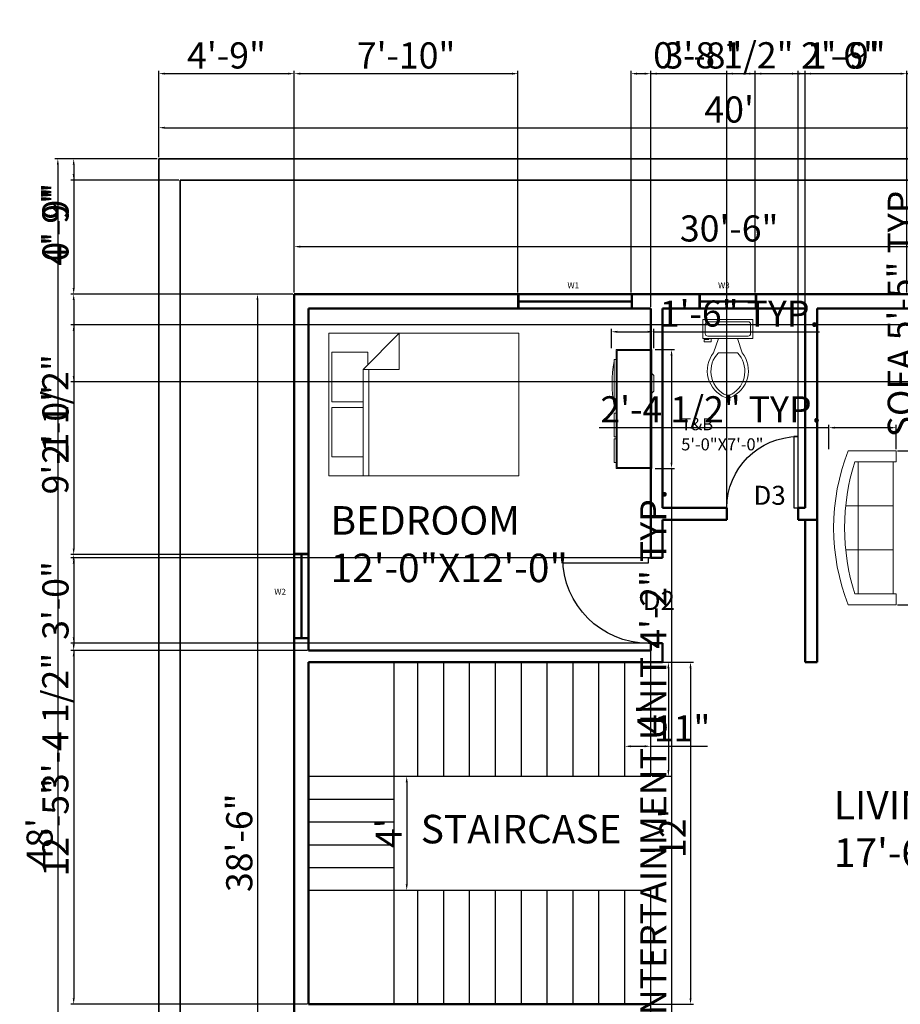
# Model space of a CAD drawing. Units: inches. Extents: x 2299 to 4423, y 1066 to 1805.
# Tile 2 of 7: x 2299 to 2670, y 1391 to 1805. Entities that reach past the tile are written whole.
import ezdxf

# ---------------------------------------------------------------- set-up
doc = ezdxf.new("R2010")
doc.units = ezdxf.units.IN
for name, color, linetype, lineweight in [('A-ANNO-DIMS', 2, 'Continuous', 18), ('A-ANNO-TEXT', 1, 'Continuous', 25), ('A-AREA-IDEN', 1, 'Continuous', 25), ('A-DOOR', 5, 'Continuous', 25), ('A-FLOR-STRS', 6, 'Continuous', 25), ('A-FURN', 8, 'Continuous', 18), ('A-GLAZ', 3, 'Continuous', 25), ('A-WALL', 7, 'Continuous', 50), ('C-PROP', 7, 'Continuous', 35)]:
    doc.layers.add(name, color=color, linetype=linetype, lineweight=lineweight)
doc.styles.get("Standard").update_dxf_attribs({"font": 'arial.ttf'})
doc.dimstyles.new('ISO-25', dxfattribs={"dimtxt": 11, "dimasz": 2.5, "dimexe": 1.25, "dimexo": 0.625, "dimtad": 1, "dimlunit": 4, "dimtxsty": 'Standard', "dimcen": 2.5, "dimadec": 0, "dimazin": 0, "dimtfac": 1, "dimtmove": 0, "dimatfit": 3, "dimfxl": 1, "dimarcsym": 0})

# ---------------------------------------------------------------- blocks, each defined once
blk = doc.blocks.new('*U2')
for p, q in [((0, 0), (0, -5)), ((30, 0), (30, -5))]:
    blk.add_line(p, q)
blk.add_lwpolyline([(0, 0), (0, 30), (1.75, 30), (1.75, 0)], close=True)
blk.add_arc((0, 0), 30, 0, 90)
blk = doc.blocks.new('Bed - Queen')
for p, q in [((0, -80.00003), (0, 0)), ((0, 0), (59.99999, 0)), ((59.99999, 0), (59.99999, -80.00003)), ((7.99999, -1.2), (28.79998, -1.2)), ((7.99999, -14.4), (7.99999, -1.2)), ((28.79998, -1.2), (28.79998, -14.4)), ((31.19999, -1.2), (51.99999, -1.2)), ((31.19999, -14.4), (31.19999, -1.2)), ((51.99999, -1.2), (51.99999, -16.4)), ((0, -14.4), (44.8, -14.4)), ((59.99999, -29.6), (44.8, -14.4)), ((44.8, -14.4), (44.8, -29.6)), ((51.99999, -16.4), (46.79936, -16.4)), ((44.8, -16.8), (0, -16.8)), ((44.8, -29.6), (59.99999, -29.6)), ((59.99999, -80.00003), (0, -80.00003))]:
    blk.add_line(p, q)
blk = doc.blocks.new('Toilet - top')
for p, q in [((9.5, -6), (9.5, -2)), ((-8, -8.5), (-8, -8)), ((-7, -8), (-7, -9.5)), ((-4, -8), (-6, -14)), ((4, -8), (6, -14)), ((-10, -8.5), (-8, -8.5)), ((-10, -9.5), (-10, -8.5)), ((-7, -9.5), (-10, -9.5)), ((4, -14), (-4, -14))]:
    blk.add_line(p, q)
blk.add_lwpolyline([(10.5, -8), (10.5, 0), (-10.5, 0), (-10.5, -8)], close=True)
for points in [[(-9.5, -2), (-9.5, -6)], [(8.5, -1), (-8.5, -1)], [(-8.5, -7), (8.5, -7)]]:
    blk.add_lwpolyline(points)
for centre, radius, start, end in [((-8.62, -1.88), 0.884, 81.8699, 188.1301), ((8.62, -1.88), 0.884, 351.8699, 98.1301), ((-8.62, -6.12), 0.884, 171.8699, 278.1301), ((8.62, -6.12), 0.884, 261.8699, 8.1301), ((3.52, -21.58), 12.17, 141.4691, 247.9714), ((4.2, -21.82), 11.33, 136.3677, 238.9468), ((-3.52, -21.58), 12.17, 292.0284, 38.5307), ((-4.2, -21.82), 11.33, 301.053, 43.6321), ((0, -27.88), 4, 245.7318, 294.2682), ((0, -29), 4, 254.8605, 285.1395)]:
    blk.add_arc(centre, radius, start, end)
blk = doc.blocks.new('Entertainment Center')
for p, q in [((-4, 0), (-5, -1)), ((4, 0), (-4, 0)), ((5, -1), (4, 0)), ((-17, -19), (-17, -1)), ((-17, -1), (43, -1)), ((-16.5, -18.5), (-16.5, -1.5)), ((-16.5, -1.5), (42.5, -1.5)), ((42.5, -1.5), (42.5, -18.5)), ((43, -1), (43, -19)), ((43, -19), (-17, -19)), ((42.5, -18.5), (-16.5, -18.5)), ((-12, -20), (-12, -19)), ((12, -19), (12, -20)), ((15, -20), (15, -19)), ((27, -19), (27, -20)), ((28, -20), (28, -19)), ((40, -19), (40, -20)), ((12, -20), (-12, -20)), ((27, -20), (15, -20)), ((40, -20), (28, -20))]:
    blk.add_line(p, q)
blk.add_arc((0, 40), 61, 259.6111, 280.3889)
blk = doc.blocks.new('Sofa - Roundback 7 ft.')
for p, q in [((-12.00002, -32.4421), (-12.00003, -6.5971)), ((11.99997, -32.4421), (11.99998, -6.5971)), ((-36.000027, -34), (-36.000027, -11.4696)), ((-35.999844, -13.3819), (35.9998, -13.3819)), ((35.99998, -34), (35.99998, -11.4696)), ((-36.000027, -32.4421), (35.99998, -32.4421))]:
    blk.add_line(p, q)
for points in [[(-36.000027, -34), (-42.000027, -34), (-42.000027, -8)], [(41.99998, -8), (41.99998, -34), (35.99998, -34)]]:
    blk.add_lwpolyline(points)
for centre, radius, start, end in [((0, -114.25), 114.25, 68.43141, 111.5686), ((-0.00001, -127.1968), 121.1968, 72.72033, 107.2797)]:
    blk.add_arc(centre, radius, start, end)
blk = doc.blocks.new('*D16')
at = {"layer": 'A-ANNO-DIMS', "color": 0, "lineweight": -2, "transparency": 16777216}
for p, q in [((2565.46, 1534.95), (2582.83, 1534.95)), ((2581.58, 1532.45), (2581.58, 1393.45)), ((2565.46, 1390.95), (2582.83, 1390.95))]:
    blk.add_line(p, q, dxfattribs=at)
at = {"layer": 'A-ANNO-DIMS', "color": 0, "transparency": 16777216}
for points in [[(2581.17, 1532.45), (2582, 1532.45), (2581.58, 1534.95)], [(2581.17, 1393.45), (2582, 1393.45), (2581.58, 1390.95)]]:
    blk.add_solid(points, dxfattribs=at)
at = {"layer": 'Defpoints', "color": 0, "transparency": 16777216}
for p in [(2564.83, 1534.95), (2564.83, 1390.95), (2581.58, 1390.95)]:
    blk.add_point(p, dxfattribs=at)
at = {"layer": 'A-ANNO-DIMS', "color": 0, "transparency": 16777216, "insert": (2575.43, 1462.95), "char_height": 11, "attachment_point": 5, "rotation": 90}
blk.add_mtext("12'", dxfattribs=at)
blk = doc.blocks.new('*D17')
at = {"layer": 'A-ANNO-DIMS', "color": 0, "lineweight": -2, "transparency": 16777216}
for p, q in [((2565.46, 1534.95), (2573.51, 1534.95)), ((2572.26, 1532.45), (2572.26, 1489.45)), ((2565.46, 1486.95), (2573.51, 1486.95))]:
    blk.add_line(p, q, dxfattribs=at)
at = {"layer": 'A-ANNO-DIMS', "color": 0, "transparency": 16777216}
for points in [[(2571.84, 1532.45), (2572.67, 1532.45), (2572.26, 1534.95)], [(2571.84, 1489.45), (2572.67, 1489.45), (2572.26, 1486.95)]]:
    blk.add_solid(points, dxfattribs=at)
at = {"layer": 'Defpoints', "color": 0, "transparency": 16777216}
for p in [(2564.83, 1534.95), (2564.83, 1486.95), (2572.26, 1486.95)]:
    blk.add_point(p, dxfattribs=at)
at = {"layer": 'A-ANNO-DIMS', "color": 0, "transparency": 16777216, "insert": (2566.13, 1510.95), "char_height": 11, "attachment_point": 5, "rotation": 90}
blk.add_mtext("4'", dxfattribs=at)
blk = doc.blocks.new('*D18')
at = {"layer": 'A-ANNO-DIMS', "color": 0, "lineweight": -2, "transparency": 16777216}
for p, q in [((2553.94, 1487.57), (2553.94, 1500.82)), ((2564.83, 1487.57), (2564.83, 1500.82)), ((2556.44, 1499.57), (2562.33, 1499.57)), ((2564.83, 1499.57), (2588.74, 1499.57))]:
    blk.add_line(p, q, dxfattribs=at)
at = {"layer": 'A-ANNO-DIMS', "color": 0, "transparency": 16777216}
for points in [[(2556.44, 1499.98), (2556.44, 1499.15), (2553.94, 1499.57)], [(2562.33, 1499.98), (2562.33, 1499.15), (2564.83, 1499.57)]]:
    blk.add_solid(points, dxfattribs=at)
at = {"layer": 'Defpoints', "color": 0, "transparency": 16777216}
for p in [(2564.83, 1499.57), (2553.94, 1486.95), (2564.83, 1486.95)]:
    blk.add_point(p, dxfattribs=at)
at = {"layer": 'A-ANNO-DIMS', "color": 0, "transparency": 16777216, "insert": (2578.04, 1505.71), "char_height": 11, "attachment_point": 5}
blk.add_mtext('11"', dxfattribs=at)
blk = doc.blocks.new('*D19')
at = {"layer": 'A-ANNO-DIMS', "color": 0, "lineweight": -2, "transparency": 16777216}
for p, q in [((2457.46, 1486.95), (2463.41, 1486.95)), ((2462.16, 1484.45), (2462.16, 1441.45)), ((2457.46, 1438.95), (2463.41, 1438.95))]:
    blk.add_line(p, q, dxfattribs=at)
at = {"layer": 'A-ANNO-DIMS', "color": 0, "transparency": 16777216}
for points in [[(2461.74, 1484.45), (2462.57, 1484.45), (2462.16, 1486.95)], [(2461.74, 1441.45), (2462.57, 1441.45), (2462.16, 1438.95)]]:
    blk.add_solid(points, dxfattribs=at)
at = {"layer": 'Defpoints', "color": 0, "transparency": 16777216}
for p in [(2456.83, 1486.95), (2456.83, 1438.95), (2462.16, 1438.95)]:
    blk.add_point(p, dxfattribs=at)
at = {"layer": 'A-ANNO-DIMS', "color": 0, "transparency": 16777216, "insert": (2456.03, 1462.95), "char_height": 11, "attachment_point": 5, "rotation": 90}
blk.add_mtext("4'", dxfattribs=at)
blk = doc.blocks.new('*D20')
at = {"layer": 'A-ANNO-DIMS', "color": 0, "lineweight": -2, "transparency": 16777216}
for p, q in [((2357.83, 1747.57), (2357.83, 1761.24)), ((2360.33, 1759.99), (2835.33, 1759.99)), ((2837.83, 1747.57), (2837.83, 1761.24))]:
    blk.add_line(p, q, dxfattribs=at)
at = {"layer": 'A-ANNO-DIMS', "color": 0, "transparency": 16777216}
for points in [[(2360.33, 1760.41), (2360.33, 1759.58), (2357.83, 1759.99)], [(2835.33, 1760.41), (2835.33, 1759.58), (2837.83, 1759.99)]]:
    blk.add_solid(points, dxfattribs=at)
at = {"layer": 'Defpoints', "color": 0, "transparency": 16777216}
for p in [(2837.83, 1759.99), (2357.83, 1746.95), (2837.83, 1746.95)]:
    blk.add_point(p, dxfattribs=at)
at = {"layer": 'A-ANNO-DIMS', "color": 0, "transparency": 16777216, "insert": (2597.83, 1766.23), "char_height": 11, "attachment_point": 5}
blk.add_mtext("40'", dxfattribs=at)
blk = doc.blocks.new('*D21')
at = {"layer": 'A-ANNO-DIMS', "color": 0, "lineweight": -2, "transparency": 16777216}
for p, q in [((2357.21, 1746.95), (2314.11, 1746.95)), ((2315.36, 1744.45), (2315.36, 1173.45)), ((2357.21, 1170.95), (2314.11, 1170.95))]:
    blk.add_line(p, q, dxfattribs=at)
at = {"layer": 'A-ANNO-DIMS', "color": 0, "transparency": 16777216}
for points in [[(2314.94, 1744.45), (2315.77, 1744.45), (2315.36, 1746.95)], [(2314.94, 1173.45), (2315.77, 1173.45), (2315.36, 1170.95)]]:
    blk.add_solid(points, dxfattribs=at)
at = {"layer": 'Defpoints', "color": 0, "transparency": 16777216}
for p in [(2357.83, 1746.95), (2315.36, 1170.95), (2357.83, 1170.95)]:
    blk.add_point(p, dxfattribs=at)
at = {"layer": 'A-ANNO-DIMS', "color": 0, "transparency": 16777216, "insert": (2309.11, 1458.95), "char_height": 11, "attachment_point": 5, "rotation": 90}
blk.add_mtext("48'", dxfattribs=at)
blk = doc.blocks.new('*D22')
at = {"layer": 'A-ANNO-DIMS', "color": 0, "lineweight": -2, "transparency": 16777216}
for p, q in [((2414.83, 1690.57), (2414.83, 1711.17)), ((2417.33, 1709.92), (2778.33, 1709.92)), ((2780.83, 1690.57), (2780.83, 1711.17))]:
    blk.add_line(p, q, dxfattribs=at)
at = {"layer": 'A-ANNO-DIMS', "color": 0, "transparency": 16777216}
for points in [[(2417.33, 1710.33), (2417.33, 1709.5), (2414.83, 1709.92)], [(2778.33, 1710.33), (2778.33, 1709.5), (2780.83, 1709.92)]]:
    blk.add_solid(points, dxfattribs=at)
at = {"layer": 'Defpoints', "color": 0, "transparency": 16777216}
for p in [(2780.83, 1709.92), (2414.83, 1689.95), (2780.83, 1689.95)]:
    blk.add_point(p, dxfattribs=at)
at = {"layer": 'A-ANNO-DIMS', "color": 0, "transparency": 16777216, "insert": (2597.83, 1716.16), "char_height": 11, "attachment_point": 5}
blk.add_mtext('30\'-6"', dxfattribs=at)
blk = doc.blocks.new('*D23')
at = {"layer": 'A-ANNO-DIMS', "color": 0, "lineweight": -2, "transparency": 16777216}
for p, q in [((2414.21, 1689.95), (2398.11, 1689.95)), ((2399.36, 1687.45), (2399.36, 1230.45)), ((2414.21, 1227.95), (2398.11, 1227.95))]:
    blk.add_line(p, q, dxfattribs=at)
at = {"layer": 'A-ANNO-DIMS', "color": 0, "transparency": 16777216}
for points in [[(2398.94, 1687.45), (2399.78, 1687.45), (2399.36, 1689.95)], [(2398.94, 1230.45), (2399.78, 1230.45), (2399.36, 1227.95)]]:
    blk.add_solid(points, dxfattribs=at)
at = {"layer": 'Defpoints', "color": 0, "transparency": 16777216}
for p in [(2414.83, 1689.95), (2399.36, 1227.95), (2414.83, 1227.95)]:
    blk.add_point(p, dxfattribs=at)
at = {"layer": 'A-ANNO-DIMS', "color": 0, "transparency": 16777216, "insert": (2393.12, 1458.95), "char_height": 11, "attachment_point": 5, "rotation": 90}
blk.add_mtext('38\'-6"', dxfattribs=at)
blk = doc.blocks.new('WIN-1200')
for p, q in [((0, 0), (0, 48.07)), ((0, 48.07), (6, 48.07)), ((0, 47.57), (6, 47.57)), ((2.8, 47.57), (2.8, 0.5)), ((3.2, 47.57), (3.2, 0.5)), ((6, 48.07), (6, 0)), ((6, 0.5), (0, 0.5)), ((6, 0), (0, 0))]:
    blk.add_line(p, q)
blk = doc.blocks.new('WIN-600')
for p, q in [((0, 6), (24.07, 6)), ((0, 0), (0, 6)), ((0.5, 0), (0.5, 6)), ((23.57, 6), (23.57, 0)), ((24.07, 6), (24.07, 0)), ((24.07, 0), (0, 0)), ((0.5, 3.2), (23.57, 3.2)), ((0.5, 2.8), (23.57, 2.8))]:
    blk.add_line(p, q)
blk = doc.blocks.new('WIN-900')
for p, q in [((0, 6), (36.07, 6)), ((0, 0), (0, 6)), ((0.5, 0), (0.5, 6)), ((35.57, 6), (35.57, 0)), ((36.07, 6), (36.07, 0)), ((36.07, 0), (0, 0)), ((0.5, 3.2), (35.57, 3.2)), ((0.5, 2.8), (35.57, 2.8))]:
    blk.add_line(p, q)
blk = doc.blocks.new('*D40')
at = {"layer": 'A-ANNO-DIMS', "color": 0, "lineweight": -2, "transparency": 16777216}
for p, q in [((2566.71, 1666.57), (2574.84, 1666.57)), ((2573.59, 1664.07), (2573.59, 1619.02)), ((2566.71, 1616.52), (2574.84, 1616.52)), ((2573.59, 1616.52), (2573.59, 1371.29))]:
    blk.add_line(p, q, dxfattribs=at)
at = {"layer": 'A-ANNO-DIMS', "color": 0, "transparency": 16777216}
for points in [[(2573.18, 1664.07), (2574.01, 1664.07), (2573.59, 1666.57)], [(2573.18, 1619.02), (2574.01, 1619.02), (2573.59, 1616.52)]]:
    blk.add_solid(points, dxfattribs=at)
at = {"layer": 'Defpoints', "color": 0, "transparency": 16777216}
for p in [(2566.08, 1666.57), (2566.08, 1616.52), (2573.59, 1616.52)]:
    blk.add_point(p, dxfattribs=at)
at = {"layer": 'A-ANNO-DIMS', "color": 0, "transparency": 16777216, "insert": (2567.35, 1492.65), "char_height": 11, "attachment_point": 5, "rotation": 90}
blk.add_mtext('ENTERTAINMENT UNIT 4\'-2" TYP.', dxfattribs=at)
blk = doc.blocks.new('*D41')
at = {"layer": 'A-ANNO-DIMS', "color": 0, "lineweight": -2, "transparency": 16777216}
for p, q in [((2548.29, 1667.2), (2548.29, 1675.33)), ((2566.08, 1667.2), (2566.08, 1675.33)), ((2550.79, 1674.08), (2563.58, 1674.08)), ((2566.08, 1674.08), (2635.85, 1674.08))]:
    blk.add_line(p, q, dxfattribs=at)
at = {"layer": 'A-ANNO-DIMS', "color": 0, "transparency": 16777216}
for points in [[(2550.79, 1674.5), (2550.79, 1673.66), (2548.29, 1674.08)], [(2563.58, 1674.5), (2563.58, 1673.66), (2566.08, 1674.08)]]:
    blk.add_solid(points, dxfattribs=at)
at = {"layer": 'Defpoints', "color": 0, "transparency": 16777216}
for p in [(2566.08, 1674.08), (2548.29, 1666.57), (2566.08, 1666.57)]:
    blk.add_point(p, dxfattribs=at)
at = {"layer": 'A-ANNO-DIMS', "color": 0, "transparency": 16777216, "insert": (2602.22, 1680.32), "char_height": 11, "attachment_point": 5}
blk.add_mtext('1\'-6" TYP.', dxfattribs=at)
blk = doc.blocks.new('*D52')
at = {"layer": 'A-ANNO-DIMS', "color": 0, "lineweight": -2, "transparency": 16777216}
for p, q in [((2677.79, 1623.96), (2677.79, 1740.82)), ((2668.68, 1623.96), (2679.04, 1623.96)), ((2677.79, 1561.58), (2677.79, 1621.46)), ((2668.68, 1559.08), (2679.04, 1559.08))]:
    blk.add_line(p, q, dxfattribs=at)
at = {"layer": 'A-ANNO-DIMS', "color": 0, "transparency": 16777216}
for points in [[(2677.37, 1621.46), (2678.21, 1621.46), (2677.79, 1623.96)], [(2677.37, 1561.58), (2678.21, 1561.58), (2677.79, 1559.08)]]:
    blk.add_solid(points, dxfattribs=at)
at = {"layer": 'Defpoints', "color": 0, "transparency": 16777216}
for p in [(2668.06, 1623.96), (2677.79, 1623.96), (2668.06, 1559.08)]:
    blk.add_point(p, dxfattribs=at)
at = {"layer": 'A-ANNO-DIMS', "color": 0, "transparency": 16777216, "insert": (2671.47, 1683.64), "char_height": 11, "attachment_point": 5, "rotation": 90}
blk.add_mtext('SOFA 5\'-5" TYP.', dxfattribs=at)
blk = doc.blocks.new('*D53')
at = {"layer": 'A-ANNO-DIMS', "color": 0, "lineweight": -2, "transparency": 16777216}
for p, q in [((2639.73, 1633.7), (2543.11, 1633.7)), ((2639.73, 1624.59), (2639.73, 1634.95)), ((2665.56, 1633.7), (2642.23, 1633.7)), ((2668.06, 1624.59), (2668.06, 1634.95))]:
    blk.add_line(p, q, dxfattribs=at)
at = {"layer": 'A-ANNO-DIMS', "color": 0, "transparency": 16777216}
for points in [[(2642.23, 1634.11), (2642.23, 1633.28), (2639.73, 1633.7)], [(2665.56, 1634.11), (2665.56, 1633.28), (2668.06, 1633.7)]]:
    blk.add_solid(points, dxfattribs=at)
at = {"layer": 'Defpoints', "color": 0, "transparency": 16777216}
for p in [(2639.73, 1633.7), (2639.73, 1623.96), (2668.06, 1623.96)]:
    blk.add_point(p, dxfattribs=at)
at = {"layer": 'A-ANNO-DIMS', "color": 0, "transparency": 16777216, "insert": (2590.17, 1640.01), "char_height": 11, "attachment_point": 5}
blk.add_mtext('2\'-4 1/2" TYP.', dxfattribs=at)
blk = doc.blocks.new('*D62')
at = {"layer": 'A-ANNO-DIMS', "color": 0, "lineweight": -2, "transparency": 16777216}
for p, q in [((2357.83, 1747.57), (2357.83, 1784)), ((2360.33, 1782.75), (2412.33, 1782.75)), ((2414.83, 1690.57), (2414.83, 1784))]:
    blk.add_line(p, q, dxfattribs=at)
at = {"layer": 'A-ANNO-DIMS', "color": 0, "transparency": 16777216}
for points in [[(2360.33, 1783.16), (2360.33, 1782.33), (2357.83, 1782.75)], [(2412.33, 1783.16), (2412.33, 1782.33), (2414.83, 1782.75)]]:
    blk.add_solid(points, dxfattribs=at)
at = {"layer": 'Defpoints', "color": 0, "transparency": 16777216}
for p in [(2414.83, 1782.75), (2357.83, 1746.95), (2414.83, 1689.95)]:
    blk.add_point(p, dxfattribs=at)
at = {"layer": 'A-ANNO-DIMS', "color": 0, "transparency": 16777216, "insert": (2386.33, 1788.99), "char_height": 11, "attachment_point": 5}
blk.add_mtext('4\'-9"', dxfattribs=at)
blk = doc.blocks.new('*D63')
at = {"layer": 'A-ANNO-DIMS', "color": 0, "lineweight": -2, "transparency": 16777216}
for p, q in [((2414.83, 1690.57), (2414.83, 1784)), ((2417.33, 1782.75), (2506.47, 1782.75)), ((2508.97, 1690.57), (2508.97, 1784))]:
    blk.add_line(p, q, dxfattribs=at)
at = {"layer": 'A-ANNO-DIMS', "color": 0, "transparency": 16777216}
for points in [[(2417.33, 1783.16), (2417.33, 1782.33), (2414.83, 1782.75)], [(2506.47, 1783.16), (2506.47, 1782.33), (2508.97, 1782.75)]]:
    blk.add_solid(points, dxfattribs=at)
at = {"layer": 'Defpoints', "color": 0, "transparency": 16777216}
for p in [(2508.97, 1782.75), (2414.83, 1689.95), (2508.97, 1689.95)]:
    blk.add_point(p, dxfattribs=at)
at = {"layer": 'A-ANNO-DIMS', "color": 0, "transparency": 16777216, "insert": (2461.9, 1788.99), "char_height": 11, "attachment_point": 5}
blk.add_mtext('7\'-10"', dxfattribs=at)
blk = doc.blocks.new('*D64')
at = {"layer": 'A-ANNO-DIMS', "color": 0, "lineweight": -2, "transparency": 16777216}
for p, q in [((2556.54, 1690.57), (2556.54, 1784)), ((2559.04, 1782.75), (2562.33, 1782.75)), ((2564.83, 1684.57), (2564.83, 1784)), ((2564.83, 1782.75), (2623.46, 1782.75))]:
    blk.add_line(p, q, dxfattribs=at)
at = {"layer": 'A-ANNO-DIMS', "color": 0, "transparency": 16777216}
for points in [[(2559.04, 1783.16), (2559.04, 1782.33), (2556.54, 1782.75)], [(2562.33, 1783.16), (2562.33, 1782.33), (2564.83, 1782.75)]]:
    blk.add_solid(points, dxfattribs=at)
at = {"layer": 'Defpoints', "color": 0, "transparency": 16777216}
for p in [(2564.83, 1782.75), (2556.54, 1689.95), (2564.83, 1683.95)]:
    blk.add_point(p, dxfattribs=at)
at = {"layer": 'A-ANNO-DIMS', "color": 0, "transparency": 16777216, "insert": (2595.39, 1789.06), "char_height": 11, "attachment_point": 5}
blk.add_mtext('0\'-8 1/2"', dxfattribs=at)
blk = doc.blocks.new('*D65')
at = {"layer": 'A-ANNO-DIMS', "color": 0, "lineweight": -2, "transparency": 16777216}
for p, q in [((2564.83, 1684.57), (2564.83, 1784)), ((2567.33, 1782.75), (2606.33, 1782.75)), ((2608.83, 1690.57), (2608.83, 1784))]:
    blk.add_line(p, q, dxfattribs=at)
at = {"layer": 'A-ANNO-DIMS', "color": 0, "transparency": 16777216}
for points in [[(2567.33, 1783.16), (2567.33, 1782.33), (2564.83, 1782.75)], [(2606.33, 1783.16), (2606.33, 1782.33), (2608.83, 1782.75)]]:
    blk.add_solid(points, dxfattribs=at)
at = {"layer": 'Defpoints', "color": 0, "transparency": 16777216}
for p in [(2608.83, 1782.75), (2608.83, 1689.95), (2564.83, 1683.95)]:
    blk.add_point(p, dxfattribs=at)
at = {"layer": 'A-ANNO-DIMS', "color": 0, "transparency": 16777216, "insert": (2586.83, 1788.99), "char_height": 11, "attachment_point": 5}
blk.add_mtext('3\'-8"', dxfattribs=at)
blk = doc.blocks.new('*D66')
at = {"layer": 'A-ANNO-DIMS', "color": 0, "lineweight": -2, "transparency": 16777216}
for p, q in [((2608.83, 1690.57), (2608.83, 1784)), ((2611.33, 1782.75), (2627.33, 1782.75)), ((2629.83, 1684.57), (2629.83, 1784)), ((2629.83, 1782.75), (2661.79, 1782.75))]:
    blk.add_line(p, q, dxfattribs=at)
at = {"layer": 'A-ANNO-DIMS', "color": 0, "transparency": 16777216}
for points in [[(2611.33, 1783.16), (2611.33, 1782.33), (2608.83, 1782.75)], [(2627.33, 1783.16), (2627.33, 1782.33), (2629.83, 1782.75)]]:
    blk.add_solid(points, dxfattribs=at)
at = {"layer": 'Defpoints', "color": 0, "transparency": 16777216}
for p in [(2629.83, 1782.75), (2608.83, 1689.95), (2629.83, 1683.95)]:
    blk.add_point(p, dxfattribs=at)
at = {"layer": 'A-ANNO-DIMS', "color": 0, "transparency": 16777216, "insert": (2647.06, 1788.99), "char_height": 11, "attachment_point": 5}
blk.add_mtext('1\'-9"', dxfattribs=at)
blk = doc.blocks.new('*D67')
at = {"layer": 'A-ANNO-DIMS', "color": 0, "lineweight": -2, "transparency": 16777216}
for p, q in [((2629.83, 1684.57), (2629.83, 1784)), ((2632.33, 1782.75), (2670.06, 1782.75)), ((2672.56, 1690.57), (2672.56, 1784)), ((2672.56, 1782.75), (2731.17, 1782.75))]:
    blk.add_line(p, q, dxfattribs=at)
at = {"layer": 'A-ANNO-DIMS', "color": 0, "transparency": 16777216}
for points in [[(2632.33, 1783.16), (2632.33, 1782.33), (2629.83, 1782.75)], [(2670.06, 1783.16), (2670.06, 1782.33), (2672.56, 1782.75)]]:
    blk.add_solid(points, dxfattribs=at)
at = {"layer": 'Defpoints', "color": 0, "transparency": 16777216}
for p in [(2672.56, 1782.75), (2672.56, 1689.95), (2629.83, 1683.95)]:
    blk.add_point(p, dxfattribs=at)
at = {"layer": 'A-ANNO-DIMS', "color": 0, "transparency": 16777216, "insert": (2703.11, 1789.06), "char_height": 11, "attachment_point": 5}
blk.add_mtext('3\'-6 1/2"', dxfattribs=at)
blk = doc.blocks.new('*D70')
at = {"layer": 'A-ANNO-DIMS', "color": 0, "lineweight": -2, "transparency": 16777216}
for p, q in [((2357.21, 1746.95), (2320.78, 1746.95)), ((2322.03, 1744.45), (2322.03, 1692.45)), ((2414.21, 1689.95), (2320.78, 1689.95))]:
    blk.add_line(p, q, dxfattribs=at)
at = {"layer": 'A-ANNO-DIMS', "color": 0, "transparency": 16777216}
for points in [[(2321.62, 1744.45), (2322.45, 1744.45), (2322.03, 1746.95)], [(2321.62, 1692.45), (2322.45, 1692.45), (2322.03, 1689.95)]]:
    blk.add_solid(points, dxfattribs=at)
at = {"layer": 'Defpoints', "color": 0, "transparency": 16777216}
for p in [(2357.83, 1746.95), (2322.03, 1689.95), (2414.83, 1689.95)]:
    blk.add_point(p, dxfattribs=at)
at = {"layer": 'A-ANNO-DIMS', "color": 0, "transparency": 16777216, "insert": (2315.79, 1718.45), "char_height": 11, "attachment_point": 5, "rotation": 90}
blk.add_mtext('4\'-9"', dxfattribs=at)
blk = doc.blocks.new('*D71')
at = {"layer": 'A-ANNO-DIMS', "color": 0, "lineweight": -2, "transparency": 16777216}
for p, q in [((2414.21, 1689.95), (2320.78, 1689.95)), ((2322.03, 1687.45), (2322.03, 1582.82)), ((2414.21, 1580.32), (2320.78, 1580.32))]:
    blk.add_line(p, q, dxfattribs=at)
at = {"layer": 'A-ANNO-DIMS', "color": 0, "transparency": 16777216}
for points in [[(2321.62, 1687.45), (2322.45, 1687.45), (2322.03, 1689.95)], [(2321.62, 1582.82), (2322.45, 1582.82), (2322.03, 1580.32)]]:
    blk.add_solid(points, dxfattribs=at)
at = {"layer": 'Defpoints', "color": 0, "transparency": 16777216}
for p in [(2414.83, 1689.95), (2322.03, 1580.32), (2414.83, 1580.32)]:
    blk.add_point(p, dxfattribs=at)
at = {"layer": 'A-ANNO-DIMS', "color": 0, "transparency": 16777216, "insert": (2315.72, 1635.13), "char_height": 11, "attachment_point": 5, "rotation": 90}
blk.add_mtext('9\'-1 1/2"', dxfattribs=at)
blk = doc.blocks.new('*D72')
at = {"layer": 'A-ANNO-DIMS', "color": 0, "lineweight": -2, "transparency": 16777216}
for p, q in [((2414.21, 1580.32), (2320.78, 1580.32)), ((2322.03, 1577.82), (2322.03, 1542.45)), ((2420.21, 1539.95), (2320.78, 1539.95)), ((2322.03, 1539.95), (2322.03, 1481.33))]:
    blk.add_line(p, q, dxfattribs=at)
at = {"layer": 'A-ANNO-DIMS', "color": 0, "transparency": 16777216}
for points in [[(2321.62, 1577.82), (2322.45, 1577.82), (2322.03, 1580.32)], [(2321.62, 1542.45), (2322.45, 1542.45), (2322.03, 1539.95)]]:
    blk.add_solid(points, dxfattribs=at)
at = {"layer": 'Defpoints', "color": 0, "transparency": 16777216}
for p in [(2414.83, 1580.32), (2322.03, 1539.95), (2420.83, 1539.95)]:
    blk.add_point(p, dxfattribs=at)
at = {"layer": 'A-ANNO-DIMS', "color": 0, "transparency": 16777216, "insert": (2315.72, 1509.39), "char_height": 11, "attachment_point": 5, "rotation": 90}
blk.add_mtext('3\'-4 1/2"', dxfattribs=at)
blk = doc.blocks.new('*D73')
at = {"layer": 'A-ANNO-DIMS', "color": 0, "lineweight": -2, "transparency": 16777216}
for p, q in [((2420.21, 1539.95), (2320.78, 1539.95)), ((2322.03, 1537.45), (2322.03, 1393.45)), ((2420.21, 1390.95), (2320.78, 1390.95))]:
    blk.add_line(p, q, dxfattribs=at)
at = {"layer": 'A-ANNO-DIMS', "color": 0, "transparency": 16777216}
for points in [[(2321.62, 1537.45), (2322.45, 1537.45), (2322.03, 1539.95)], [(2321.62, 1393.45), (2322.45, 1393.45), (2322.03, 1390.95)]]:
    blk.add_solid(points, dxfattribs=at)
at = {"layer": 'Defpoints', "color": 0, "transparency": 16777216}
for p in [(2420.83, 1539.95), (2322.03, 1390.95), (2420.83, 1390.95)]:
    blk.add_point(p, dxfattribs=at)
at = {"layer": 'A-ANNO-DIMS', "color": 0, "transparency": 16777216, "insert": (2315.79, 1465.45), "char_height": 11, "attachment_point": 5, "rotation": 90}
blk.add_mtext('12\'-5"', dxfattribs=at)
blk = doc.blocks.new('*D77')
at = {"layer": 'A-ANNO-DIMS', "color": 0, "lineweight": -2, "transparency": 16777216}
for p, q in [((2357.21, 1746.95), (2320.78, 1746.95)), ((2322.03, 1744.45), (2322.03, 1740.45)), ((2366.21, 1737.95), (2320.78, 1737.95)), ((2322.03, 1737.95), (2322.03, 1704.95))]:
    blk.add_line(p, q, dxfattribs=at)
at = {"layer": 'A-ANNO-DIMS', "color": 0, "transparency": 16777216}
for points in [[(2321.62, 1744.45), (2322.45, 1744.45), (2322.03, 1746.95)], [(2321.62, 1740.45), (2322.45, 1740.45), (2322.03, 1737.95)]]:
    blk.add_solid(points, dxfattribs=at)
at = {"layer": 'Defpoints', "color": 0, "transparency": 16777216}
for p in [(2357.83, 1746.95), (2322.03, 1737.95), (2366.83, 1737.95)]:
    blk.add_point(p, dxfattribs=at)
at = {"layer": 'A-ANNO-DIMS', "color": 0, "transparency": 16777216, "insert": (2315.79, 1720.2), "char_height": 11, "attachment_point": 5, "rotation": 90}
blk.add_mtext('0\'-9"', dxfattribs=at)
blk = doc.blocks.new('*D88')
at = {"layer": 'A-ANNO-DIMS', "color": 0, "lineweight": -2, "transparency": 16777216}
for p, q in [((2596.83, 1595.57), (2596.83, 1784)), ((2599.33, 1782.75), (2624.33, 1782.75)), ((2626.83, 1595.57), (2626.83, 1784)), ((2626.83, 1782.75), (2660.01, 1782.75))]:
    blk.add_line(p, q, dxfattribs=at)
at = {"layer": 'A-ANNO-DIMS', "color": 0, "transparency": 16777216}
for points in [[(2599.33, 1783.16), (2599.33, 1782.33), (2596.83, 1782.75)], [(2624.33, 1783.16), (2624.33, 1782.33), (2626.83, 1782.75)]]:
    blk.add_solid(points, dxfattribs=at)
at = {"layer": 'Defpoints', "color": 0, "transparency": 16777216}
for p in [(2626.83, 1782.75), (2596.83, 1594.95), (2626.83, 1594.95)]:
    blk.add_point(p, dxfattribs=at)
at = {"layer": 'A-ANNO-DIMS', "color": 0, "transparency": 16777216, "insert": (2644.67, 1788.99), "char_height": 11, "attachment_point": 5}
blk.add_mtext('2\'-6"', dxfattribs=at)
blk = doc.blocks.new('*D89')
at = {"layer": 'A-ANNO-DIMS', "color": 0, "lineweight": -2, "transparency": 16777216}
for p, q in [((2738.21, 1676.95), (2320.78, 1676.95)), ((2322.03, 1674.45), (2322.03, 1655.45)), ((2738.21, 1652.95), (2320.78, 1652.95)), ((2322.03, 1652.95), (2322.03, 1619.77))]:
    blk.add_line(p, q, dxfattribs=at)
at = {"layer": 'A-ANNO-DIMS', "color": 0, "transparency": 16777216}
for points in [[(2321.62, 1674.45), (2322.45, 1674.45), (2322.03, 1676.95)], [(2321.62, 1655.45), (2322.45, 1655.45), (2322.03, 1652.95)]]:
    blk.add_solid(points, dxfattribs=at)
at = {"layer": 'Defpoints', "color": 0, "transparency": 16777216}
for p in [(2738.83, 1676.95), (2322.03, 1652.95), (2738.83, 1652.95)]:
    blk.add_point(p, dxfattribs=at)
at = {"layer": 'A-ANNO-DIMS', "color": 0, "transparency": 16777216, "insert": (2315.79, 1635.11), "char_height": 11, "attachment_point": 5, "rotation": 90}
blk.add_mtext('2\'-0"', dxfattribs=at)
blk = doc.blocks.new('*D90')
at = {"layer": 'A-ANNO-DIMS', "color": 0, "lineweight": -2, "transparency": 16777216}
for p, q in [((2569.21, 1578.95), (2320.78, 1578.95)), ((2322.03, 1576.45), (2322.03, 1545.45)), ((2569.21, 1542.95), (2320.78, 1542.95))]:
    blk.add_line(p, q, dxfattribs=at)
at = {"layer": 'A-ANNO-DIMS', "color": 0, "transparency": 16777216}
for points in [[(2321.62, 1576.45), (2322.45, 1576.45), (2322.03, 1578.95)], [(2321.62, 1545.45), (2322.45, 1545.45), (2322.03, 1542.95)]]:
    blk.add_solid(points, dxfattribs=at)
at = {"layer": 'Defpoints', "color": 0, "transparency": 16777216}
for p in [(2569.83, 1578.95), (2322.03, 1542.95), (2569.83, 1542.95)]:
    blk.add_point(p, dxfattribs=at)
at = {"layer": 'A-ANNO-DIMS', "color": 0, "transparency": 16777216, "insert": (2315.79, 1560.95), "char_height": 11, "attachment_point": 5, "rotation": 90}
blk.add_mtext('3\'-0"', dxfattribs=at)

msp = doc.modelspace()

# ---------------------------------------------------------------- linework, layer by layer
at = {"layer": 'A-FLOR-STRS'}
for p, q in [((2564.834, 1486.945), (2564.834, 1539.945)), ((2456.834, 1534.945), (2420.834, 1534.945)), ((2420.834, 1534.945), (2420.834, 1390.945)), ((2456.834, 1390.945), (2456.834, 1534.945)), ((2466.834, 1486.945), (2466.834, 1534.945)), ((2477.723, 1486.945), (2477.723, 1534.945)), ((2488.611, 1486.945), (2488.611, 1534.945)), ((2499.5, 1486.945), (2499.5, 1534.945)), ((2510.389, 1486.945), (2510.389, 1534.945)), ((2521.278, 1486.945), (2521.278, 1534.945)), ((2532.167, 1486.945), (2532.167, 1534.945)), ((2543.056, 1486.945), (2543.056, 1534.945)), ((2553.945, 1486.945), (2553.945, 1534.945)), ((2564.834, 1486.945), (2564.834, 1534.945)), ((2420.834, 1486.945), (2564.834, 1486.945)), ((2420.834, 1477.345), (2456.834, 1477.345)), ((2420.834, 1467.745), (2456.834, 1467.745)), ((2420.834, 1458.145), (2456.834, 1458.145)), ((2420.834, 1448.545), (2456.834, 1448.545)), ((2420.834, 1438.945), (2564.834, 1438.945)), ((2420.834, 1438.945), (2564.834, 1438.945)), ((2466.834, 1390.945), (2466.834, 1438.945)), ((2477.723, 1390.945), (2477.723, 1438.945)), ((2488.611, 1390.945), (2488.611, 1438.945)), ((2499.5, 1390.945), (2499.5, 1438.945)), ((2510.389, 1390.945), (2510.389, 1438.945)), ((2521.278, 1390.945), (2521.278, 1438.945)), ((2532.167, 1390.945), (2532.167, 1438.945)), ((2543.056, 1390.945), (2543.056, 1438.945)), ((2553.945, 1390.945), (2553.945, 1438.945)), ((2564.834, 1390.945), (2564.834, 1438.945)), ((2564.834, 1385.945), (2564.834, 1438.945)), ((2420.834, 1390.945), (2456.834, 1390.945))]:
    msp.add_line(p, q, dxfattribs=at)
at = {"layer": 'A-WALL'}
for p, q in [((2414.834, 1227.945), (2414.834, 1689.945)), ((2414.834, 1689.945), (2780.834, 1689.945)), ((2420.834, 1683.945), (2564.834, 1683.945)), ((2420.834, 1539.945), (2420.834, 1683.945)), ((2564.834, 1578.945), (2564.834, 1683.945)), ((2569.834, 1683.945), (2629.834, 1683.945)), ((2569.834, 1599.945), (2569.834, 1683.945)), ((2629.834, 1599.945), (2629.834, 1683.945)), ((2634.834, 1594.945), (2634.834, 1683.945)), ((2634.834, 1683.945), (2774.834, 1683.945)), ((2569.834, 1599.945), (2596.834, 1599.945)), ((2596.834, 1599.945), (2596.834, 1594.945)), ((2626.834, 1594.945), (2626.834, 1599.945)), ((2626.834, 1599.945), (2629.834, 1599.945)), ((2569.834, 1594.945), (2596.834, 1594.945)), ((2569.834, 1578.945), (2569.834, 1594.945)), ((2634.834, 1594.945), (2626.834, 1594.945)), ((2626.834, 1594.945), (2629.834, 1594.945)), ((2629.834, 1594.945), (2629.834, 1534.945)), ((2634.834, 1594.945), (2634.834, 1534.945)), ((2564.834, 1578.945), (2569.834, 1578.945)), ((2564.834, 1539.945), (2564.834, 1542.945)), ((2569.834, 1542.945), (2564.834, 1542.945)), ((2569.834, 1534.945), (2569.834, 1542.945)), ((2569.834, 1539.945), (2569.834, 1542.945)), ((2420.834, 1539.945), (2564.834, 1539.945)), ((2420.834, 1534.945), (2569.834, 1534.945)), ((2420.834, 1390.945), (2420.834, 1534.945)), ((2634.834, 1534.945), (2629.834, 1534.945)), ((2420.834, 1390.945), (2564.834, 1390.945))]:
    msp.add_line(p, q, dxfattribs=at)
at = {"layer": 'C-PROP'}
for p, q in [((2357.834, 1170.945), (2357.834, 1746.945)), ((2357.834, 1746.945), (2837.834, 1746.945)), ((2366.834, 1737.945), (2828.834, 1737.945)), ((2366.834, 1179.945), (2366.834, 1737.945))]:
    msp.add_line(p, q, dxfattribs=at)

# ---------------------------------------------------------------- block references
at = {"layer": 'A-DOOR', "xscale": -1}
msp.add_blockref('*U2', (2626.834, 1599.945), dxfattribs=at)
at = {"layer": 'A-DOOR', "xscale": -1.199999999999999, "yscale": 1.199999999999999, "zscale": 1.199999999999999, "rotation": 90}
msp.add_blockref('*U2', (2563.834, 1578.945), dxfattribs=at)
at = {"layer": 'A-FURN'}
msp.add_blockref('Toilet - top', (2597.297, 1679.277), dxfattribs=at)
at = {"layer": 'A-FURN', "rotation": 90}
msp.add_blockref('Bed - Queen', (2429.387, 1613.448), dxfattribs=at)
at = {"layer": 'A-FURN'}
for name, p, xscale, yscale, zscale, rotation in [('Entertainment Center', (2566.085, 1652.392), 0.8342103315264846, 0.8342103315264846, 0.8342103315264846, 270), ('Sofa - Roundback 7 ft.', (2641.794, 1591.523), 0.7724308018975573, 0.7724308018975573, 0.7724308018975573, 90)]:
    msp.add_blockref(name, p, dxfattribs=dict(at, xscale=xscale, yscale=yscale, zscale=zscale, rotation=rotation))
at = {"layer": 'A-GLAZ'}
for name, p, rotation in [('WIN-1200', (2557.037, 1683.945), 90.00000000000014), ('WIN-900', (2414.833, 1580.816), 269.9999999999987)]:
    msp.add_blockref(name, p, dxfattribs=dict(at, rotation=rotation))
msp.add_blockref('WIN-600', (2585.261, 1683.945), dxfattribs=at)

# ---------------------------------------------------------------- texts
at = {"layer": 'A-ANNO-TEXT', "char_height": 2.5, "attachment_point": 1}
for s, insert in [('W1', (2529.805, 1694.855)), ('W3', (2593.183, 1694.855)), ('W2', (2406.458, 1565.902))]:
    msp.add_mtext(s, dxfattribs=dict(at, insert=insert))
at = {"layer": 'A-ANNO-TEXT', "char_height": 8, "attachment_point": 1}
for s, insert in [('D3', (2608.079, 1609.228)), ('D2', (2561.47, 1564.924))]:
    msp.add_mtext_dynamic_manual_height_columns(s, width=1.11117, gutter_width=12.5, heights=[0], dxfattribs=dict(at, insert=insert))
at = {"layer": 'A-AREA-IDEN', "attachment_point": 1}
for s, width, gutter_width, insert, char_height in [('T&B\\P5\'-0"X7\'-0"', 2.46662, 25.4, (2577.659, 1637.696), 5.07992), ('BEDROOM\\P12\'-0"X12\'-0"', 9.28623, 12.5, (2430.105, 1600.672), 12), ('LIVINGROOM\\P17\'-6"X14\'-8"', 12, 12.5, (2641.889, 1480.805), 12), ('STAIRCASE', 9.28623, 12.5, (2468.07, 1470.702), 12)]:
    msp.add_mtext_dynamic_manual_height_columns(s, width=width, gutter_width=gutter_width, heights=[0], dxfattribs=dict(at, insert=insert, char_height=char_height))

# ---------------------------------------------------------------- dimensions: what is measured, and where the dimension line sits
at = {"layer": 'A-ANNO-DIMS'}
for base, p1, p2, override, picture, middle in [((2564.834, 1782.745), (2556.537, 1689.945), (2564.834, 1683.945), {"dimdec": 1, "dimlfac": 1, "dimrnd": 0, "dimzin": 1, "dimdsep": 46, "dimlunit": 4, "dimfrac": 2}, '*D64', (2595.395, 1789.058)), ((2672.556, 1782.745), (2629.834, 1683.945), (2672.556, 1689.945), {"dimdec": 1, "dimlfac": 1, "dimrnd": 0, "dimzin": 1, "dimdsep": 46, "dimlunit": 4, "dimfrac": 2}, '*D67', (2703.114, 1789.062)), ((2414.834, 1782.745), (2357.834, 1746.945), (2414.834, 1689.945), {"dimdec": 1, "dimlfac": 1, "dimrnd": 0, "dimzin": 1, "dimdsep": 46, "dimlunit": 4, "dimfrac": 2}, '*D62', (2386.334, 1788.987)), ((2508.966, 1782.745), (2414.834, 1689.945), (2508.966, 1689.945), {"dimdec": 1, "dimlfac": 1, "dimrnd": 0, "dimzin": 1, "dimdsep": 46, "dimlunit": 4, "dimfrac": 2}, '*D63', (2461.9, 1788.987)), ((2608.832, 1782.745), (2564.834, 1683.945), (2608.832, 1689.945), {"dimdec": 1, "dimlfac": 1, "dimrnd": 0, "dimzin": 1, "dimdsep": 46, "dimlunit": 4, "dimfrac": 2}, '*D65', (2586.833, 1788.99)), ((2626.834, 1782.745), (2596.834, 1594.945), (2626.834, 1594.945), {"dimdec": 1, "dimlfac": 1, "dimrnd": 0, "dimzin": 1, "dimdsep": 46, "dimlunit": 4, "dimfrac": 2}, '*D88', (2644.673, 1788.987)), ((2629.834, 1782.745), (2608.832, 1689.945), (2629.834, 1683.945), {"dimdec": 1, "dimlfac": 1, "dimrnd": 0, "dimzin": 1, "dimdsep": 46, "dimlunit": 4, "dimfrac": 2}, '*D66', (2647.061, 1788.987)), ((2837.834, 1759.993), (2357.834, 1746.945), (2837.834, 1746.945), {"dimclrd": 0, "dimclre": 0, "dimclrt": 0}, '*D20', (2597.834, 1766.235)), ((2780.834, 1709.917), (2414.834, 1689.945), (2780.834, 1689.945), {"dimclrd": 0, "dimclre": 0, "dimclrt": 0}, '*D22', (2597.834, 1716.162)), ((2564.834, 1499.565), (2553.945, 1486.945), (2564.834, 1486.945), {"dimclrd": 0, "dimclre": 0, "dimclrt": 0}, '*D18', (2578.036, 1505.713))]:
    dim = msp.add_linear_dim(base=base, p1=p1, p2=p2, dimstyle='ISO-25', override=override, dxfattribs=at)
    dim.commit()
    dim.dimension.update_dxf_attribs({"geometry": picture, "text_midpoint": middle})
for base, p1, p2, override, picture, middle in [((2315.355, 1170.945), (2357.834, 1746.945), (2357.834, 1170.945), {"dimclrd": 0, "dimclre": 0, "dimclrt": 0}, '*D21', (2309.114, 1458.945)), ((2322.034, 1689.945), (2357.834, 1746.945), (2414.834, 1689.945), {"dimdec": 1, "dimlfac": 1, "dimrnd": 0, "dimzin": 1, "dimdsep": 46, "dimlunit": 4, "dimfrac": 2}, '*D70', (2315.792, 1718.445)), ((2322.034, 1737.945), (2357.834, 1746.945), (2366.834, 1737.945), {"dimdec": 1, "dimlfac": 1, "dimrnd": 0, "dimzin": 1, "dimdsep": 46, "dimlunit": 4, "dimfrac": 2}, '*D77', (2315.792, 1720.2)), ((2322.034, 1580.315), (2414.834, 1689.945), (2414.834, 1580.315), {"dimdec": 1, "dimlfac": 1, "dimrnd": 0, "dimzin": 1, "dimdsep": 46, "dimlunit": 4, "dimfrac": 2}, '*D71', (2315.721, 1635.13)), ((2399.361, 1227.945), (2414.834, 1689.945), (2414.834, 1227.945), {"dimclrd": 0, "dimclre": 0, "dimclrt": 0}, '*D23', (2393.116, 1458.945)), ((2322.034, 1652.945), (2738.834, 1676.945), (2738.834, 1652.945), {"dimdec": 1, "dimlfac": 1, "dimrnd": 0, "dimzin": 1, "dimdsep": 46, "dimlunit": 4, "dimfrac": 2}, '*D89', (2315.792, 1635.106)), ((2322.034, 1539.945), (2414.834, 1580.315), (2420.834, 1539.945), {"dimdec": 1, "dimlfac": 1, "dimrnd": 0, "dimzin": 1, "dimdsep": 46, "dimlunit": 4, "dimfrac": 2}, '*D72', (2315.717, 1509.388)), ((2322.034, 1542.945), (2569.834, 1578.945), (2569.834, 1542.945), {"dimdec": 1, "dimlfac": 1, "dimrnd": 0, "dimzin": 1, "dimdsep": 46, "dimlunit": 4, "dimfrac": 2}, '*D90', (2315.789, 1560.945)), ((2322.034, 1390.945), (2420.834, 1539.945), (2420.834, 1390.945), {"dimdec": 1, "dimlfac": 1, "dimrnd": 0, "dimzin": 1, "dimdsep": 46, "dimlunit": 4, "dimfrac": 2}, '*D73', (2315.792, 1465.445)), ((2572.257, 1486.945), (2564.834, 1534.945), (2564.834, 1486.945), {"dimclrd": 0, "dimclre": 0, "dimclrt": 0}, '*D17', (2566.132, 1510.945)), ((2581.582, 1390.945), (2564.834, 1534.945), (2564.834, 1390.945), {"dimclrd": 0, "dimclre": 0, "dimclrt": 0}, '*D16', (2575.435, 1462.945)), ((2462.155, 1438.945), (2456.834, 1486.945), (2456.834, 1438.945), {"dimclrd": 0, "dimclre": 0, "dimclrt": 0}, '*D19', (2456.03, 1462.945))]:
    dim = msp.add_linear_dim(base=base, p1=p1, p2=p2, angle=90, dimstyle='ISO-25', override=override, dxfattribs=at)
    dim.commit()
    dim.dimension.update_dxf_attribs({"geometry": picture, "text_midpoint": middle})
for base, p1, p2, angle, text, picture, middle in [((2677.789, 1623.965), (2668.057, 1559.081), (2668.057, 1623.965), 90, 'SOFA <> TYP.', '*D52', (2671.473, 1683.643)), ((2573.593, 1616.521), (2566.085, 1666.573), (2566.085, 1616.521), 270, 'ENTERTAINMENT UNIT <> TYP.', '*D40', (2567.352, 1492.655)), ((2639.734, 1633.697), (2668.057, 1623.965), (2639.734, 1623.965), 180, '<> TYP.', '*D53', (2590.174, 1640.01))]:
    dim = msp.add_linear_dim(base=base, p1=p1, p2=p2, angle=angle, text=text, dimstyle='ISO-25', override={"dimdec": 1, "dimrnd": 0, "dimzin": 1, "dimlunit": 4, "dimfrac": 2}, dxfattribs=at)
    dim.commit()
    dim.dimension.update_dxf_attribs({"geometry": picture, "text_midpoint": middle})
dim = msp.add_linear_dim(base=(2566.085, 1674.081), p1=(2548.289, 1666.573), p2=(2566.085, 1666.573), text='<> TYP.', dimstyle='ISO-25', override={"dimdec": 1, "dimrnd": 0, "dimzin": 1, "dimlunit": 4, "dimfrac": 2}, dxfattribs=at)
dim.commit()
dim.dimension.update_dxf_attribs({"geometry": '*D41', "text_midpoint": (2602.217, 1680.323)})

doc.saveas('drawing.dxf')
